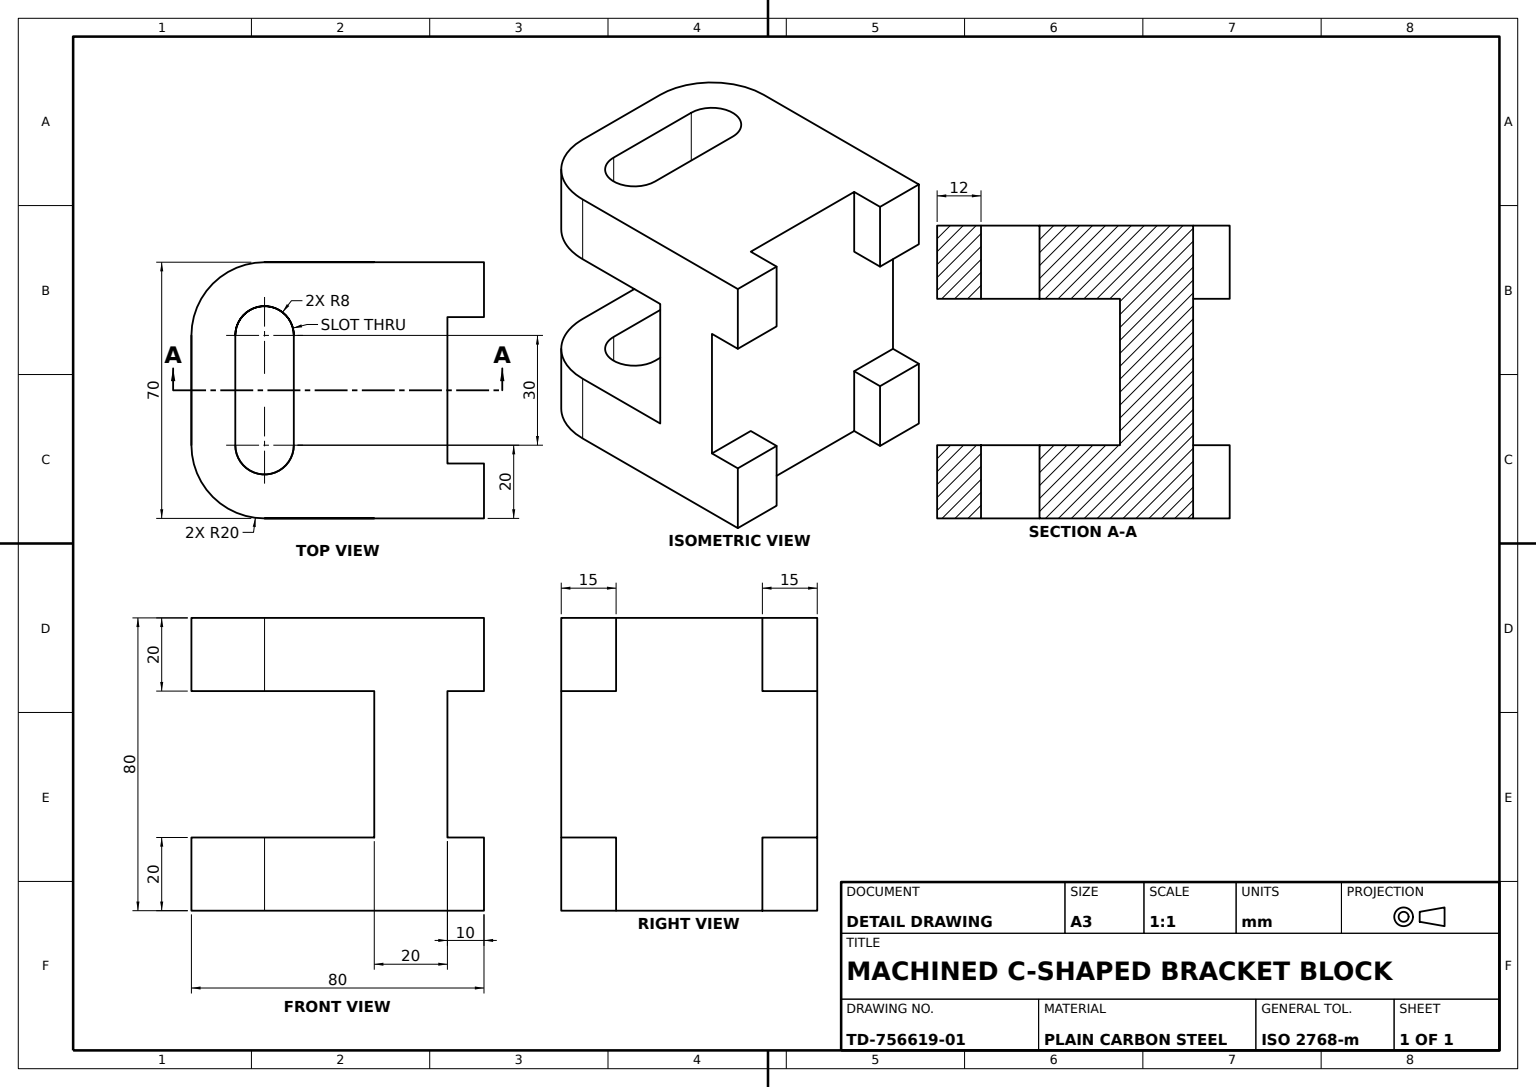
from build123d import *

# Parameters (mm, degrees)
BASE_PLATE_SKETCH_W          = 70
BASE_PLATE_SKETCH_H          = 70
BASE_PLATE_70X70_DEPTH       = 20
WEB_BLOCK_SKETCH_W           = 15
WEB_BLOCK_SKETCH_H           = 10
WEB_BLOCK_DEPTH              = 25
SIDE_BLOCK_A_SKETCH_W        = 15
SIDE_BLOCK_A_SKETCH_H        = 10
SIDE_BLOCK_A_DEPTH           = 25
SIDE_BLOCK_B_SKETCH_W        = 15
SIDE_BLOCK_B_SKETCH_H        = 10
SIDE_BLOCK_B_DEPTH           = 25
POCKET_CUT_A_SKETCH_W        = 10
POCKET_CUT_A_SKETCH_H        = 10
POCKET_CUT_A_DEPTH           = 70
POCKET_CUT_B_SKETCH_W        = 10
POCKET_CUT_B_SKETCH_H        = 10
POCKET_CUT_B_DEPTH           = 70
FLANGE_A_5MM_DEPTH           = 5
FLANGE_B_5MM_DEPTH           = 5
ROUNDED_TAB_A_DEPTH          = 20
ROUNDED_START                = -20
ROUNDED_TAB_B_DEPTH          = 20
TAB_SLOTS_8X30_THROUGH_DEPTH = 80


with BuildPart() as part:
    # Base Plate Sketch → Base Plate 70x70 (new body)
    with BuildSketch(Plane.XY):
        with Locations((35, 35)):
            Rectangle(BASE_PLATE_SKETCH_W, BASE_PLATE_SKETCH_H)
    extrude(amount=BASE_PLATE_70X70_DEPTH)

    # Web Block Sketch → Web Block (add)
    with BuildSketch(Plane.XZ):
        with Locations((7.5, -5)):
            Rectangle(WEB_BLOCK_SKETCH_W, WEB_BLOCK_SKETCH_H)
        with Locations((62.5, -5)):
            Rectangle(WEB_BLOCK_SKETCH_W, WEB_BLOCK_SKETCH_H)
    extrude(amount=-WEB_BLOCK_DEPTH)

    # Side Block A Sketch → Side Block A (add)
    with BuildSketch(Plane(origin=(0, 70, 0), x_dir=(1, 0, 0), z_dir=(0, 1, 0))):
        with Locations((7.5, 5)):
            Rectangle(SIDE_BLOCK_A_SKETCH_W, SIDE_BLOCK_A_SKETCH_H)
    extrude(amount=-SIDE_BLOCK_A_DEPTH)

    # Side Block B Sketch → Side Block B (add)
    with BuildSketch(Plane(origin=(0, 70, 0), x_dir=(1, 0, 0), z_dir=(0, 1, 0))):
        with Locations((62.5, 5)):
            Rectangle(SIDE_BLOCK_B_SKETCH_W, SIDE_BLOCK_B_SKETCH_H)
    extrude(amount=-SIDE_BLOCK_B_DEPTH)

    # Pocket Cut A Sketch → Pocket Cut A (cut)
    with BuildSketch(Plane(origin=(70, 0, 0), x_dir=(0, 0, -1), z_dir=(1, 0, 0))):
        with Locations((5, 50)):
            Rectangle(POCKET_CUT_A_SKETCH_W, POCKET_CUT_A_SKETCH_H)
    extrude(amount=-POCKET_CUT_A_DEPTH, mode=Mode.SUBTRACT)

    # Pocket Cut B Sketch → Pocket Cut B (cut)
    with BuildSketch(Plane(origin=(70, 0, 0), x_dir=(0, 0, -1), z_dir=(1, 0, 0))):
        with Locations((5, 20)):
            Rectangle(POCKET_CUT_B_SKETCH_W, POCKET_CUT_B_SKETCH_H)
    extrude(amount=-POCKET_CUT_B_DEPTH, mode=Mode.SUBTRACT)

    # Flange A Sketch → Flange A 5mm (add)
    with BuildSketch(Plane.XZ):
        Polygon((0, 20), (70, 20), (70, -10), (55, -10), (55, 0), (15, 0), (15, -10), (0, -10), align=None)
    extrude(amount=FLANGE_A_5MM_DEPTH)

    # Flange B Sketch → Flange B 5mm (add)
    with BuildSketch(Plane(origin=(0, 70, 0), x_dir=(1, 0, 0), z_dir=(0, 1, 0))):
        Polygon((0, -20), (70, -20), (70, 10), (55, 10), (55, 0), (15, 0), (15, 10), (0, 10), align=None)
    extrude(amount=FLANGE_B_5MM_DEPTH)

    # Rounded Tab A Sketch → Rounded Tab A (add)
    with BuildSketch(Plane.XZ.offset(5)):
        with BuildLine():
            Line((0, 20), (0, 50))
            ThreePointArc((0, 50), (5.857864376, 64.142135624), (20, 70))
            Line((20, 70), (50, 70))
            ThreePointArc((50, 70), (64.142135624, 64.142135624), (70, 50))
            Line((70, 50), (70, 20))
            Line((70, 20), (0, 20))
        make_face()
    extrude(amount=-ROUNDED_TAB_A_DEPTH)

    # Rounded Tab B Sketch → Rounded Tab B (add)
    with BuildSketch(Plane(origin=(0, 75, 0), x_dir=(1, 0, 0), z_dir=(0, 1, 0)).offset(ROUNDED_START)):
        with BuildLine():
            Line((0, -20), (0, -50))
            ThreePointArc((0, -50), (5.857864376, -64.142135624), (20, -70))
            Line((20, -70), (50, -70))
            ThreePointArc((50, -70), (64.142135624, -64.142135624), (70, -50))
            Line((70, -50), (70, -20))
            Line((70, -20), (0, -20))
        make_face()
    extrude(amount=ROUNDED_TAB_B_DEPTH)

    # Tab Slots Sketch → Tab Slots 8x30 Through (cut)
    with BuildSketch(Plane.XZ.offset(5)):
        with BuildLine():
            Line((20, 58), (50, 58))
            ThreePointArc((50, 58), (58, 50), (50, 42))
            Line((50, 42), (20, 42))
            ThreePointArc((20, 42), (12, 50), (20, 58))
        make_face()
    extrude(amount=-TAB_SLOTS_8X30_THROUGH_DEPTH, mode=Mode.SUBTRACT)


solid = part.part
